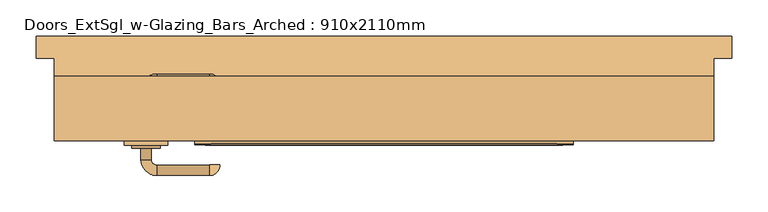
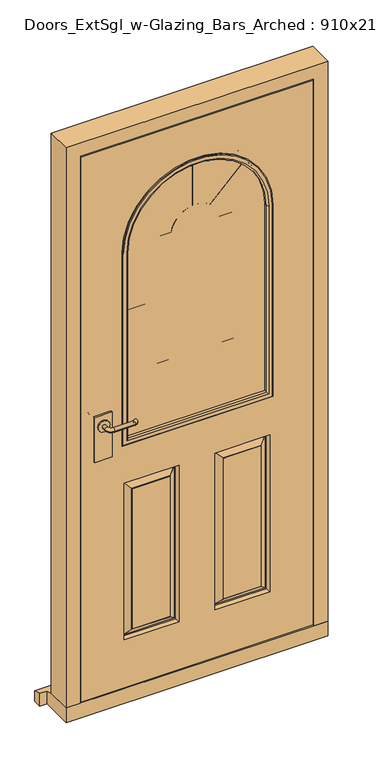
"""IFC4 building model written with IfcOpenShell, lengths in millimetres: door geometry, Doors_ExtSgl_w-Glazing_Bars_Arched : 910x2110mm."""

from ifc_helpers import new_model, si_unit, point, frame, frame_2d, origin, place, context, project, spatial, polyline, circle_curve, ellipse_curve, trimmed, segment, composite_curve, outline, extrude, faceted_brep, source, transform, mapped, element, save
from ifc_brep_helpers import plane_surface, cylinder_surface, revolved_surface, advanced_brep


def doors_extsgl_w_glazing_bars_arched_910x2110mm_1ab485ba(model_context):
    return source(origin(), model_context, "Body", "SolidModel", [
        extrude(outline(composite_curve([segment(trimmed(circle_curve(frame_2d((1050.0, -328.5)), 20.0), [point((1050.0, -348.5))], [point((1050.0, -308.5))], False, "CARTESIAN"), True, "CONTINUOUS"), segment(trimmed(circle_curve(frame_2d((1050.0, -328.5)), 20.0), [point((1050.0, -308.5))], [point((1050.0, -348.5))], False, "CARTESIAN"), True, "CONTINUOUS")], self_intersect=False)), frame((0.0, -22.9929895, 0.0), z_axis=(0.0, 1.0, 0.0), x_axis=(0.0, 0.0, 1.0)), (0.0, 0.0, 1.0), 4.5929895),
        advanced_brep(
        [(-321.5, -22.9929895, 1050.0), (-335.5, -22.9929895, 1050.0), (-335.5, -38.4, 1050.0), (-321.5, -38.4, 1050.0), (-313.5, -60.4, 1050.0), (-313.5, -46.4, 1050.0), (-241.5, -60.4, 1050.0), (-241.5, -46.4, 1050.0), (-240.5, -45.4, 1050.0), (-226.5, -45.4, 1050.0)],
        [
            (0, 1, circle_curve(frame((-328.5, -22.9929895, 1050.0), z_axis=(0.0, 1.0, 0.0), x_axis=(-1.0, 0.0, 0.0)), 7.0)),
            (1, 0, circle_curve(frame((-328.5, -22.9929895, 1050.0), z_axis=(0.0, 1.0, 0.0), x_axis=(-1.0, 0.0, 0.0)), 7.0)),
            (1, 2),
            (2, 3, circle_curve(frame((-328.5, -38.4, 1050.0), z_axis=(0.0, 1.0, 0.0), x_axis=(-1.0, 0.0, 0.0)), 7.0)),
            (3, 0),
            (3, 2, circle_curve(frame((-328.5, -38.4, 1050.0), z_axis=(0.0, 1.0, 0.0), x_axis=(-1.0, 0.0, 0.0)), 7.0)),
            (4, 5, circle_curve(frame((-313.5, -53.4, 1050.0), z_axis=(-1.0, 0.0, 0.0), x_axis=(0.0, -1.0, 0.0)), 7.0)),
            (5, 3, circle_curve(frame((-313.5, -38.4, 1050.0), z_axis=(0.0, 0.0, -1.0), x_axis=(-1.0, 0.0, 0.0)), 8.0)),
            (2, 4, circle_curve(frame((-313.5, -38.4, 1050.0), z_axis=(0.0, 0.0, 1.0), x_axis=(-1.0, 0.0, 0.0)), 22.0)),
            (5, 4, circle_curve(frame((-313.5, -53.4, 1050.0), z_axis=(-1.0, 0.0, 0.0), x_axis=(0.0, -1.0, 0.0)), 7.0)),
            (4, 6),
            (6, 7, circle_curve(frame((-241.5, -53.4, 1050.0), z_axis=(-1.0, 0.0, 0.0), x_axis=(0.0, -1.0, 0.0)), 7.0)),
            (7, 5),
            (7, 6, circle_curve(frame((-241.5, -53.4, 1050.0), z_axis=(-1.0, 0.0, 0.0), x_axis=(0.0, -1.0, 0.0)), 7.0)),
            (8, 9, circle_curve(frame((-233.5, -45.4, 1050.0), z_axis=(0.0, 1.0, 0.0), x_axis=(1.0, 0.0, 0.0)), 7.0)),
            (9, 8, circle_curve(frame((-233.5, -45.4, 1050.0), z_axis=(0.0, 1.0, 0.0), x_axis=(1.0, 0.0, 0.0)), 7.0)),
            (8, 7, circle_curve(frame((-241.5, -45.4, 1050.0), z_axis=(0.0, 0.0, -1.0), x_axis=(0.0, -1.0, 0.0)), 1.0)),
            (6, 9, circle_curve(frame((-241.5, -45.4, 1050.0), z_axis=(0.0, 0.0, 1.0), x_axis=(0.0, -1.0, 0.0)), 15.0)),
        ],
        [
            plane_surface(frame((-328.5, -22.9929895, 1050.0), z_axis=(0.0, 1.0, 0.0), x_axis=(0.0, 0.0, 1.0))),
            cylinder_surface(frame((-328.5, -22.9929895, 1050.0), z_axis=(0.0, 1.0, 0.0), x_axis=(-1.0, 0.0, 0.0)), 7.0),
            revolved_surface(trimmed(ellipse_curve(frame((-328.5, -38.4, 1050.0), z_axis=(0.0, -1.0, 0.0), x_axis=(-1.0, 0.0, 0.0)), 7.0, 7.0), [point((-321.5, -38.4, 1050.0))], [point((-335.5, -38.4, 1050.0))], True, "CARTESIAN"), (-313.5, -38.4, 1050.0), (0.0, 0.0, -1.0)),
            revolved_surface(trimmed(ellipse_curve(frame((-328.5, -38.4, 1050.0), z_axis=(0.0, -1.0, 0.0), x_axis=(-1.0, 0.0, 0.0)), 7.0, 7.0), [point((-335.5, -38.4, 1050.0))], [point((-321.5, -38.4, 1050.0))], True, "CARTESIAN"), (-313.5, -38.4, 1050.0), (0.0, 0.0, -1.0)),
            cylinder_surface(frame((-313.5, -53.4, 1050.0), z_axis=(-1.0, 0.0, 0.0), x_axis=(0.0, -1.0, 0.0)), 7.0),
            plane_surface(frame((-233.5, -45.4, 1050.0), z_axis=(0.0, 1.0, 0.0), x_axis=(0.0, 0.0, 1.0))),
            revolved_surface(trimmed(ellipse_curve(frame((-241.5, -53.4, 1050.0), z_axis=(1.0, 0.0, 0.0), x_axis=(0.0, -1.0, 0.0)), 7.0, 7.0), [point((-241.5, -46.4, 1050.0))], [point((-241.5, -60.4, 1050.0))], True, "CARTESIAN"), (-241.5, -45.4, 1050.0), (0.0, 0.0, -1.0)),
            revolved_surface(trimmed(ellipse_curve(frame((-241.5, -53.4, 1050.0), z_axis=(1.0, 0.0, 0.0), x_axis=(0.0, -1.0, 0.0)), 7.0, 7.0), [point((-241.5, -60.4, 1050.0))], [point((-241.5, -46.4, 1050.0))], True, "CARTESIAN"), (-241.5, -45.4, 1050.0), (0.0, 0.0, -1.0)),
        ],
        [
            (0, [[1, 2]]),
            (1, [[3, 4, 5, -2]]),
            (1, [[-5, 6, -3, -1]]),
            (2, [[7, 8, -4, 9]]),
            (3, [[10, -9, -6, -8]]),
            (4, [[11, 12, 13, -7]]),
            (4, [[-13, 14, -11, -10]]),
            (5, [[15, 16]]),
            (6, [[-15, 17, -12, 18]]),
            (7, [[-16, -18, -14, -17]]),
        ],
    ),
        extrude(outline(polyline([(-298.5, -12.4), (-298.5, -18.4), (-358.5, -18.4), (-358.5, -12.4), (-298.5, -12.4)])), frame((0.0, 0.0, 925.0), z_axis=(0.0, 0.0, 1.0), x_axis=(1.0, 0.0, 0.0)), (0.0, 0.0, 1.0), 165.0),
        extrude(outline(composite_curve([segment(trimmed(circle_curve(frame_2d((1050.0, -328.5)), 20.0), [point((1050.0, -348.5))], [point((1050.0, -308.5))], False, "CARTESIAN"), True, "CONTINUOUS"), segment(trimmed(circle_curve(frame_2d((1050.0, -328.5)), 20.0), [point((1050.0, -308.5))], [point((1050.0, -348.5))], False, "CARTESIAN"), True, "CONTINUOUS")], self_intersect=False)), frame((0.0, 37.6, 0.0), z_axis=(0.0, 1.0, 0.0), x_axis=(0.0, 0.0, 1.0)), (0.0, 0.0, 1.0), 4.5929895),
        advanced_brep(
        [(-321.5, 42.1929895, 1050.0), (-335.5, 42.1929895, 1050.0), (-321.5, 57.6, 1050.0), (-335.5, 57.6, 1050.0), (-313.5, 79.6, 1050.0), (-313.5, 65.6, 1050.0), (-241.5, 65.6, 1050.0), (-241.5, 79.6, 1050.0), (-240.5, 64.6, 1050.0), (-226.5, 64.6, 1050.0)],
        [
            (0, 1, circle_curve(frame((-328.5, 42.1929895, 1050.0), z_axis=(0.0, -1.0, 0.0), x_axis=(-1.0, 0.0, 0.0)), 7.0)),
            (1, 0, circle_curve(frame((-328.5, 42.1929895, 1050.0), z_axis=(0.0, -1.0, 0.0), x_axis=(-1.0, 0.0, 0.0)), 7.0)),
            (0, 2),
            (2, 3, circle_curve(frame((-328.5, 57.6, 1050.0), z_axis=(0.0, -1.0, 0.0), x_axis=(-1.0, 0.0, 0.0)), 7.0)),
            (3, 1),
            (3, 2, circle_curve(frame((-328.5, 57.6, 1050.0), z_axis=(0.0, -1.0, 0.0), x_axis=(-1.0, 0.0, 0.0)), 7.0)),
            (4, 3, circle_curve(frame((-313.5, 57.6, 1050.0), z_axis=(0.0, 0.0, 1.0), x_axis=(-1.0, 0.0, 0.0)), 22.0)),
            (2, 5, circle_curve(frame((-313.5, 57.6, 1050.0), z_axis=(0.0, 0.0, -1.0), x_axis=(-1.0, 0.0, 0.0)), 8.0)),
            (5, 4, circle_curve(frame((-313.5, 72.6, 1050.0), z_axis=(-1.0, 0.0, 0.0), x_axis=(0.0, 1.0, 0.0)), 7.0)),
            (4, 5, circle_curve(frame((-313.5, 72.6, 1050.0), z_axis=(-1.0, 0.0, 0.0), x_axis=(0.0, 1.0, 0.0)), 7.0)),
            (5, 6),
            (6, 7, circle_curve(frame((-241.5, 72.6, 1050.0), z_axis=(-1.0, 0.0, 0.0), x_axis=(0.0, 1.0, 0.0)), 7.0)),
            (7, 4),
            (7, 6, circle_curve(frame((-241.5, 72.6, 1050.0), z_axis=(-1.0, 0.0, 0.0), x_axis=(0.0, 1.0, 0.0)), 7.0)),
            (8, 9, circle_curve(frame((-233.5, 64.6, 1050.0), z_axis=(0.0, -1.0, 0.0), x_axis=(1.0, 0.0, 0.0)), 7.0)),
            (9, 8, circle_curve(frame((-233.5, 64.6, 1050.0), z_axis=(0.0, -1.0, 0.0), x_axis=(1.0, 0.0, 0.0)), 7.0)),
            (9, 7, circle_curve(frame((-241.5, 64.6, 1050.0), z_axis=(0.0, 0.0, 1.0), x_axis=(0.0, 1.0, 0.0)), 15.0)),
            (6, 8, circle_curve(frame((-241.5, 64.6, 1050.0), z_axis=(0.0, 0.0, -1.0), x_axis=(0.0, 1.0, 0.0)), 1.0)),
        ],
        [
            plane_surface(frame((-328.5, 42.1929895, 1050.0), z_axis=(0.0, -1.0, 0.0), x_axis=(0.0, 0.0, 1.0))),
            cylinder_surface(frame((-328.5, 42.1929895, 1050.0), z_axis=(0.0, -1.0, 0.0), x_axis=(-1.0, 0.0, 0.0)), 7.0),
            revolved_surface(trimmed(ellipse_curve(frame((-328.5, 57.6, 1050.0), z_axis=(0.0, -1.0, 0.0), x_axis=(-1.0, 0.0, 0.0)), 7.0, 7.0), [point((-321.5, 57.6, 1050.0))], [point((-335.5, 57.6, 1050.0))], True, "CARTESIAN"), (-313.5, 57.6, 1050.0), (0.0, 0.0, -1.0)),
            revolved_surface(trimmed(ellipse_curve(frame((-328.5, 57.6, 1050.0), z_axis=(0.0, -1.0, 0.0), x_axis=(-1.0, 0.0, 0.0)), 7.0, 7.0), [point((-335.5, 57.6, 1050.0))], [point((-321.5, 57.6, 1050.0))], True, "CARTESIAN"), (-313.5, 57.6, 1050.0), (0.0, 0.0, -1.0)),
            cylinder_surface(frame((-313.5, 72.6, 1050.0), z_axis=(-1.0, 0.0, 0.0), x_axis=(0.0, 1.0, 0.0)), 7.0),
            plane_surface(frame((-233.5, 64.6, 1050.0), z_axis=(0.0, -1.0, 0.0), x_axis=(0.0, 0.0, 1.0))),
            revolved_surface(trimmed(ellipse_curve(frame((-241.5, 72.6, 1050.0), z_axis=(-1.0, 0.0, 0.0), x_axis=(0.0, 1.0, 0.0)), 7.0, 7.0), [point((-241.5, 65.6, 1050.0))], [point((-241.5, 79.6, 1050.0))], True, "CARTESIAN"), (-241.5, 64.6, 1050.0), (0.0, 0.0, -1.0)),
            revolved_surface(trimmed(ellipse_curve(frame((-241.5, 72.6, 1050.0), z_axis=(-1.0, 0.0, 0.0), x_axis=(0.0, 1.0, 0.0)), 7.0, 7.0), [point((-241.5, 79.6, 1050.0))], [point((-241.5, 65.6, 1050.0))], True, "CARTESIAN"), (-241.5, 64.6, 1050.0), (0.0, 0.0, -1.0)),
        ],
        [
            (0, [[1, 2]]),
            (1, [[-1, 3, 4, 5]]),
            (1, [[-2, -5, 6, -3]]),
            (2, [[7, -4, 8, 9]]),
            (3, [[-8, -6, -7, 10]]),
            (4, [[-9, 11, 12, 13]]),
            (4, [[-10, -13, 14, -11]]),
            (5, [[15, 16]]),
            (6, [[17, -12, 18, -16]]),
            (7, [[-18, -14, -17, -15]]),
        ],
    ),
        extrude(outline(polyline([(-298.5, 31.6), (-358.5, 31.6), (-358.5, 37.6), (-298.5, 37.6), (-298.5, 31.6)])), frame((0.0, 0.0, 925.0), z_axis=(0.0, 0.0, 1.0), x_axis=(1.0, 0.0, 0.0)), (0.0, 0.0, 1.0), 165.0),
        faceted_brep([(384.5, 76.6, 54.5), (455.0, 76.6, 54.5), (455.0, -12.4, 54.5), (406.5, -12.4, 54.5), (406.5, 34.6, 54.5), (384.5, 34.6, 54.5), (384.5, 76.6, 2039.5), (-384.5, 76.6, 2039.5), (-384.5, 76.6, 54.5), (-455.0, 76.6, 54.5), (-455.0, 76.6, 2110.0), (455.0, 76.6, 2110.0), (455.0, -12.4, 2110.0), (-455.0, -12.4, 2110.0), (-455.0, -12.4, 54.5), (-406.5, -12.4, 54.5), (-406.5, -12.4, 2061.5), (406.5, -12.4, 2061.5), (406.5, 34.6, 2061.5), (-406.5, 34.6, 2061.5), (-406.5, 34.6, 54.5), (-384.5, 34.6, 54.5), (-384.5, 34.6, 2039.5), (384.5, 34.6, 2039.5)], [[[0, 1, 2, 3, 4, 5]], [[1, 0, 6, 7, 8, 9, 10, 11]], [[2, 1, 11, 12]], [[3, 2, 12, 13, 14, 15, 16, 17]], [[4, 3, 17, 18]], [[5, 4, 18, 19, 20, 21, 22, 23]], [[0, 5, 23, 6]], [[8, 7, 22, 21]], [[9, 8, 21, 20, 15, 14]], [[10, 9, 14, 13]], [[16, 15, 20, 19]], [[11, 10, 13, 12]], [[17, 16, 19, 18]], [[7, 6, 23, 22]]]),
        advanced_brep(
        [(403.5, -12.4, 58.5), (403.5, -12.4, 2058.5), (-404.4250294, -12.4, 2058.5), (-404.4250294, -12.4, 58.5), (-253.5, -12.4, 958.5), (-253.5, -12.4, 1655.0), (253.5, -12.4, 1655.0), (253.5, -12.4, 958.5), (-62.5, -12.4, 808.5), (-62.5, -12.4, 233.5), (-253.5, -12.4, 233.5), (-253.5, -12.4, 808.5), (253.5, -12.4, 808.5), (253.5, -12.4, 233.5), (62.5, -12.4, 233.5), (62.5, -12.4, 808.5), (-92.5, -12.4, 263.5), (-92.5, -12.4, 778.5), (-223.5, -12.4, 778.5), (-223.5, -12.4, 263.5), (223.5, -12.4, 263.5), (223.5, -12.4, 778.5), (92.5, -12.4, 778.5), (92.5, -12.4, 263.5), (403.5, 31.6, 58.5), (-404.4250294, 31.6, 58.5), (-404.4250294, 31.6, 2058.5), (403.5, 31.6, 2058.5), (-253.5, 31.6, 958.5), (253.5, 31.6, 958.5), (253.5, 31.6, 1655.0), (-253.5, 31.6, 1655.0), (62.5, 31.6, 808.5), (62.5, 31.6, 233.5), (253.5, 31.6, 233.5), (253.5, 31.6, 808.5), (-253.5, 31.6, 808.5), (-253.5, 31.6, 233.5), (-62.5, 31.6, 233.5), (-62.5, 31.6, 808.5), (92.5, 31.6, 263.5), (92.5, 31.6, 778.5), (223.5, 31.6, 778.5), (223.5, 31.6, 263.5), (-223.5, 31.6, 263.5), (-223.5, 31.6, 778.5), (-92.5, 31.6, 778.5), (-92.5, 31.6, 263.5), (65.5, 16.6, 805.5), (65.5, 16.6, 236.5), (90.5, 30.6, 780.5), (90.5, 30.6, 261.5), (70.5, 16.6, 241.5), (70.5, 16.6, 800.5), (92.5, 30.6, 263.5), (92.5, 30.6, 778.5), (250.5, 16.6, 236.5), (225.5, 30.6, 261.5), (245.5, 16.6, 241.5), (223.5, 30.6, 263.5), (250.5, 16.6, 805.5), (225.5, 30.6, 780.5), (245.5, 16.6, 800.5), (223.5, 30.6, 778.5), (-250.5, 16.6, 805.5), (-250.5, 16.6, 236.5), (-225.5, 30.6, 780.5), (-225.5, 30.6, 261.5), (-245.5, 16.6, 241.5), (-245.5, 16.6, 800.5), (-223.5, 30.6, 263.5), (-223.5, 30.6, 778.5), (-65.5, 16.6, 236.5), (-90.5, 30.6, 261.5), (-70.5, 16.6, 241.5), (-92.5, 30.6, 263.5), (-65.5, 16.6, 805.5), (-90.5, 30.6, 780.5), (-70.5, 16.6, 800.5), (-92.5, 30.6, 778.5), (-92.5, -11.4, 263.5), (-92.5, -11.4, 778.5), (-70.5, 2.6, 241.5), (-70.5, 2.6, 800.5), (-90.5, -11.4, 780.5), (-90.5, -11.4, 261.5), (-65.5, 2.6, 805.5), (-65.5, 2.6, 236.5), (-223.5, -11.4, 778.5), (-245.5, 2.6, 800.5), (-225.5, -11.4, 780.5), (-250.5, 2.6, 805.5), (-223.5, -11.4, 263.5), (-245.5, 2.6, 241.5), (-225.5, -11.4, 261.5), (-250.5, 2.6, 236.5), (250.5, 2.6, 805.5), (250.5, 2.6, 236.5), (225.5, -11.4, 780.5), (225.5, -11.4, 261.5), (245.5, 2.6, 241.5), (245.5, 2.6, 800.5), (223.5, -11.4, 263.5), (223.5, -11.4, 778.5), (65.5, 2.6, 236.5), (90.5, -11.4, 261.5), (70.5, 2.6, 241.5), (92.5, -11.4, 263.5), (65.5, 2.6, 805.5), (90.5, -11.4, 780.5), (70.5, 2.6, 800.5), (92.5, -11.4, 778.5)],
        [
            (0, 1),
            (1, 2),
            (2, 3),
            (3, 0),
            (4, 5),
            (5, 6, circle_curve(frame((0.0, -12.4, 1655.0), z_axis=(0.0, 1.0, 0.0), x_axis=(1.0, 0.0, 0.0)), 253.5)),
            (6, 7),
            (7, 4),
            (8, 9),
            (9, 10),
            (10, 11),
            (11, 8),
            (12, 13),
            (13, 14),
            (14, 15),
            (15, 12),
            (16, 17),
            (17, 18),
            (18, 19),
            (19, 16),
            (20, 21),
            (21, 22),
            (22, 23),
            (23, 20),
            (24, 25),
            (25, 26),
            (26, 27),
            (27, 24),
            (28, 29),
            (29, 30),
            (30, 31, circle_curve(frame((0.0, 31.6, 1655.0), z_axis=(0.0, -1.0, 0.0), x_axis=(1.0, 0.0, 0.0)), 253.5)),
            (31, 28),
            (32, 33),
            (33, 34),
            (34, 35),
            (35, 32),
            (36, 37),
            (37, 38),
            (38, 39),
            (39, 36),
            (40, 41),
            (41, 42),
            (42, 43),
            (43, 40),
            (44, 45),
            (45, 46),
            (46, 47),
            (47, 44),
            (0, 24),
            (27, 1),
            (26, 2),
            (25, 3),
            (4, 28),
            (31, 5),
            (30, 6),
            (29, 7),
            (48, 49),
            (49, 33),
            (32, 48),
            (50, 51),
            (51, 52),
            (52, 53),
            (53, 50),
            (40, 54),
            (54, 55),
            (55, 41),
            (49, 56),
            (56, 34),
            (51, 57),
            (57, 58),
            (58, 52),
            (43, 59),
            (59, 54),
            (56, 60),
            (60, 35),
            (57, 61),
            (61, 62),
            (62, 58),
            (42, 63),
            (63, 59),
            (60, 48),
            (62, 53),
            (61, 50),
            (63, 55),
            (64, 65),
            (65, 37),
            (36, 64),
            (66, 67),
            (67, 68),
            (68, 69),
            (69, 66),
            (44, 70),
            (70, 71),
            (71, 45),
            (65, 72),
            (72, 38),
            (67, 73),
            (73, 74),
            (74, 68),
            (47, 75),
            (75, 70),
            (72, 76),
            (76, 39),
            (73, 77),
            (77, 78),
            (78, 74),
            (46, 79),
            (79, 75),
            (76, 64),
            (78, 69),
            (77, 66),
            (79, 71),
            (80, 81),
            (81, 17),
            (16, 80),
            (82, 83),
            (83, 84),
            (84, 85),
            (85, 82),
            (8, 86),
            (86, 87),
            (87, 9),
            (81, 88),
            (88, 18),
            (83, 89),
            (89, 90),
            (90, 84),
            (11, 91),
            (91, 86),
            (88, 92),
            (92, 19),
            (89, 93),
            (93, 94),
            (94, 90),
            (10, 95),
            (95, 91),
            (92, 80),
            (94, 85),
            (93, 82),
            (95, 87),
            (96, 97),
            (97, 13),
            (12, 96),
            (98, 99),
            (99, 100),
            (100, 101),
            (101, 98),
            (20, 102),
            (102, 103),
            (103, 21),
            (97, 104),
            (104, 14),
            (99, 105),
            (105, 106),
            (106, 100),
            (23, 107),
            (107, 102),
            (104, 108),
            (108, 15),
            (105, 109),
            (109, 110),
            (110, 106),
            (22, 111),
            (111, 107),
            (108, 96),
            (110, 101),
            (109, 98),
            (111, 103),
        ],
        [
            plane_surface(frame((403.5, -12.4, 58.5), z_axis=(0.0, -1.0, 0.0), x_axis=(0.0, 0.0, 1.0))),
            plane_surface(frame((403.5, 31.6, 58.5), z_axis=(0.0, 1.0, 0.0), x_axis=(0.0, 0.0, -1.0))),
            plane_surface(frame((403.5, -12.4, 58.5), z_axis=(1.0, 0.0, 0.0), x_axis=(0.0, 1.0, 0.0))),
            plane_surface(frame((403.5, -12.4, 2058.5), z_axis=(0.0, 0.0, 1.0), x_axis=(0.0, 1.0, 0.0))),
            plane_surface(frame((-404.4250294, -12.4, 2058.5), z_axis=(-1.0, 0.0, 0.0), x_axis=(0.0, 1.0, 0.0))),
            plane_surface(frame((-404.4250294, -12.4, 58.5), z_axis=(0.0, 0.0, -1.0), x_axis=(0.0, 1.0, 0.0))),
            plane_surface(frame((-253.5, -12.4, 958.5), z_axis=(1.0, 0.0, 0.0), x_axis=(0.0, 1.0, 0.0))),
            revolved_surface(polyline([(253.5, 31.6, 1655.0), (253.5, -12.4, 1655.0)]), (0.0, -12.4, 1655.0), (0.0, 1.0, 0.0)),
            plane_surface(frame((253.5, -12.4, 1655.0), z_axis=(-1.0, 0.0, 0.0), x_axis=(0.0, 1.0, 0.0))),
            plane_surface(frame((253.5, -12.4, 958.5), z_axis=(0.0, 0.0, 1.0), x_axis=(0.0, 1.0, 0.0))),
            plane_surface(frame((62.5, 31.6, 808.5), z_axis=(0.9805806756909202, 0.19611613513818407, 0.0), x_axis=(0.0, 0.0, -1.0))),
            plane_surface(frame((70.5, 16.6, 800.5), z_axis=(-0.5734623443633278, 0.8192319205190408, 0.0), x_axis=(0.0, 0.0, -1.0))),
            plane_surface(frame((92.5, 30.6, 778.5), z_axis=(-1.0, 0.0, 0.0), x_axis=(0.0, 0.0, -1.0))),
            plane_surface(frame((62.5, 31.6, 233.5), z_axis=(0.0, 0.19611613513818724, 0.9805806756909196), x_axis=(1.0, 0.0, 0.0))),
            plane_surface(frame((70.5, 16.6, 241.5), z_axis=(0.0, 0.819231920519039, -0.5734623443633305), x_axis=(1.0, 0.0, 0.0))),
            plane_surface(frame((92.5, 30.6, 263.5), z_axis=(0.0, 0.0, -1.0), x_axis=(1.0, 0.0, 0.0))),
            plane_surface(frame((253.5, 31.6, 233.5), z_axis=(-0.9805806756909189, 0.19611613513819037, 0.0), x_axis=(0.0, 0.0, 1.0))),
            plane_surface(frame((245.5, 16.6, 241.5), z_axis=(0.5734623443633332, 0.819231920519037, 0.0), x_axis=(0.0, 0.0, 1.0))),
            plane_surface(frame((223.5, 30.6, 263.5), z_axis=(1.0, 0.0, 0.0), x_axis=(0.0, 0.0, 1.0))),
            plane_surface(frame((253.5, 31.6, 808.5), z_axis=(0.0, 0.1961161351381872, -0.9805806756909196), x_axis=(-1.0, 0.0, 0.0))),
            plane_surface(frame((250.5, 16.6, 805.5), z_axis=(0.0, 1.0, 0.0), x_axis=(-1.0, 0.0, 0.0))),
            plane_surface(frame((245.5, 16.6, 800.5), z_axis=(0.0, 0.8192319205190389, 0.5734623443633305), x_axis=(-1.0, 0.0, 0.0))),
            plane_surface(frame((225.5, 30.6, 780.5), z_axis=(0.0, 1.0, 0.0), x_axis=(-1.0, 0.0, 0.0))),
            plane_surface(frame((223.5, 30.6, 778.5), z_axis=(0.0, 0.0, 1.0), x_axis=(-1.0, 0.0, 0.0))),
            plane_surface(frame((-253.5, 31.6, 808.5), z_axis=(0.9805806756909202, 0.19611613513818407, 0.0), x_axis=(0.0, 0.0, -1.0))),
            plane_surface(frame((-245.5, 16.6, 800.5), z_axis=(-0.5734623443633278, 0.8192319205190408, 0.0), x_axis=(0.0, 0.0, -1.0))),
            plane_surface(frame((-223.5, 30.6, 778.5), z_axis=(-1.0, 0.0, 0.0), x_axis=(0.0, 0.0, -1.0))),
            plane_surface(frame((-253.5, 31.6, 233.5), z_axis=(0.0, 0.19611613513818724, 0.9805806756909196), x_axis=(1.0, 0.0, 0.0))),
            plane_surface(frame((-245.5, 16.6, 241.5), z_axis=(0.0, 0.819231920519039, -0.5734623443633305), x_axis=(1.0, 0.0, 0.0))),
            plane_surface(frame((-223.5, 30.6, 263.5), z_axis=(0.0, 0.0, -1.0), x_axis=(1.0, 0.0, 0.0))),
            plane_surface(frame((-62.5, 31.6, 233.5), z_axis=(-0.9805806756909189, 0.1961161351381904, 0.0), x_axis=(0.0, 0.0, 1.0))),
            plane_surface(frame((-70.5, 16.6, 241.5), z_axis=(0.5734623443633332, 0.8192319205190371, 0.0), x_axis=(0.0, 0.0, 1.0))),
            plane_surface(frame((-92.5, 30.6, 263.5), z_axis=(1.0, 0.0, 0.0), x_axis=(0.0, 0.0, 1.0))),
            plane_surface(frame((-62.5, 31.6, 808.5), z_axis=(0.0, 0.19611613513818724, -0.9805806756909196), x_axis=(-1.0, 0.0, 0.0))),
            plane_surface(frame((-65.5, 16.6, 805.5), z_axis=(0.0, 1.0, 0.0), x_axis=(-1.0, 0.0, 0.0))),
            plane_surface(frame((-70.5, 16.6, 800.5), z_axis=(0.0, 0.819231920519039, 0.5734623443633305), x_axis=(-1.0, 0.0, 0.0))),
            plane_surface(frame((-90.5, 30.6, 780.5), z_axis=(0.0, 1.0, 0.0), x_axis=(-1.0, 0.0, 0.0))),
            plane_surface(frame((-92.5, 30.6, 778.5), z_axis=(0.0, 0.0, 1.0), x_axis=(-1.0, 0.0, 0.0))),
            plane_surface(frame((-92.5, -12.4, 263.5), z_axis=(1.0, 0.0, 0.0), x_axis=(0.0, 0.0, 1.0))),
            plane_surface(frame((-90.5, -11.4, 261.5), z_axis=(0.5734623443633226, -0.8192319205190446, 0.0), x_axis=(0.0, 0.0, 1.0))),
            plane_surface(frame((-65.5, 2.6, 236.5), z_axis=(-0.9805806756909214, -0.19611613513817774, 0.0), x_axis=(0.0, 0.0, 1.0))),
            plane_surface(frame((-92.5, -12.4, 778.5), z_axis=(0.0, 0.0, 1.0), x_axis=(-1.0, 0.0, 0.0))),
            plane_surface(frame((-90.5, -11.4, 780.5), z_axis=(0.0, -0.8192319205190427, 0.5734623443633252), x_axis=(-1.0, 0.0, 0.0))),
            plane_surface(frame((-65.5, 2.6, 805.5), z_axis=(0.0, -0.1961161351381809, -0.9805806756909208), x_axis=(-1.0, 0.0, 0.0))),
            plane_surface(frame((-223.5, -12.4, 778.5), z_axis=(-1.0, 0.0, 0.0), x_axis=(0.0, 0.0, -1.0))),
            plane_surface(frame((-225.5, -11.4, 780.5), z_axis=(-0.5734623443633279, -0.8192319205190408, 0.0), x_axis=(0.0, 0.0, -1.0))),
            plane_surface(frame((-250.5, 2.6, 805.5), z_axis=(0.9805806756909202, -0.1961161351381841, 0.0), x_axis=(0.0, 0.0, -1.0))),
            plane_surface(frame((-223.5, -12.4, 263.5), z_axis=(0.0, 0.0, -1.0), x_axis=(1.0, 0.0, 0.0))),
            plane_surface(frame((-223.5, -11.4, 263.5), z_axis=(0.0, -1.0, 0.0), x_axis=(1.0, 0.0, 0.0))),
            plane_surface(frame((-225.5, -11.4, 261.5), z_axis=(0.0, -0.8192319205190427, -0.5734623443633252), x_axis=(1.0, 0.0, 0.0))),
            plane_surface(frame((-245.5, 2.6, 241.5), z_axis=(0.0, -1.0, 0.0), x_axis=(1.0, 0.0, 0.0))),
            plane_surface(frame((-250.5, 2.6, 236.5), z_axis=(0.0, -0.19611613513818094, 0.9805806756909209), x_axis=(1.0, 0.0, 0.0))),
            plane_surface(frame((253.5, -12.4, 808.5), z_axis=(-0.9805806756909202, -0.19611613513818407, 0.0), x_axis=(0.0, 0.0, -1.0))),
            plane_surface(frame((245.5, 2.6, 800.5), z_axis=(0.5734623443633278, -0.8192319205190408, 0.0), x_axis=(0.0, 0.0, -1.0))),
            plane_surface(frame((223.5, -11.4, 778.5), z_axis=(1.0, 0.0, 0.0), x_axis=(0.0, 0.0, -1.0))),
            plane_surface(frame((253.5, -12.4, 233.5), z_axis=(0.0, -0.19611613513818724, 0.9805806756909196), x_axis=(-1.0, 0.0, 0.0))),
            plane_surface(frame((245.5, 2.6, 241.5), z_axis=(0.0, -0.819231920519039, -0.5734623443633305), x_axis=(-1.0, 0.0, 0.0))),
            plane_surface(frame((223.5, -11.4, 263.5), z_axis=(0.0, 0.0, -1.0), x_axis=(-1.0, 0.0, 0.0))),
            plane_surface(frame((62.5, -12.4, 233.5), z_axis=(0.9805806756909189, -0.19611613513819046, 0.0), x_axis=(0.0, 0.0, 1.0))),
            plane_surface(frame((70.5, 2.6, 241.5), z_axis=(-0.5734623443633331, -0.8192319205190371, 0.0), x_axis=(0.0, 0.0, 1.0))),
            plane_surface(frame((92.5, -11.4, 263.5), z_axis=(-1.0, 0.0, 0.0), x_axis=(0.0, 0.0, 1.0))),
            plane_surface(frame((62.5, -12.4, 808.5), z_axis=(0.0, -0.1961161351381873, -0.9805806756909196), x_axis=(1.0, 0.0, 0.0))),
            plane_surface(frame((65.5, 2.6, 805.5), z_axis=(0.0, -1.0, 0.0), x_axis=(1.0, 0.0, 0.0))),
            plane_surface(frame((70.5, 2.6, 800.5), z_axis=(0.0, -0.819231920519039, 0.5734623443633304), x_axis=(1.0, 0.0, 0.0))),
            plane_surface(frame((90.5, -11.4, 780.5), z_axis=(0.0, -1.0, 0.0), x_axis=(1.0, 0.0, 0.0))),
            plane_surface(frame((92.5, -11.4, 778.5), z_axis=(0.0, 0.0, 1.0), x_axis=(1.0, 0.0, 0.0))),
        ],
        [
            (0, [[1, 2, 3, 4], [5, 6, 7, 8], [9, 10, 11, 12], [13, 14, 15, 16]]),
            (0, [[17, 18, 19, 20]]),
            (0, [[21, 22, 23, 24]]),
            (1, [[25, 26, 27, 28], [29, 30, 31, 32], [33, 34, 35, 36], [37, 38, 39, 40]]),
            (1, [[41, 42, 43, 44]]),
            (1, [[45, 46, 47, 48]]),
            (2, [[-1, 49, -28, 50]]),
            (3, [[-2, -50, -27, 51]]),
            (4, [[-3, -51, -26, 52]]),
            (5, [[-4, -52, -25, -49]]),
            (6, [[-5, 53, -32, 54]]),
            (7, [[-6, -54, -31, 55]]),
            (8, [[-7, -55, -30, 56]]),
            (9, [[-8, -56, -29, -53]]),
            (10, [[57, 58, -33, 59]]),
            (11, [[60, 61, 62, 63]]),
            (12, [[64, 65, 66, -41]]),
            (13, [[-58, 67, 68, -34]]),
            (14, [[-61, 69, 70, 71]]),
            (15, [[-64, -44, 72, 73]]),
            (16, [[-68, 74, 75, -35]]),
            (17, [[-70, 76, 77, 78]]),
            (18, [[-72, -43, 79, 80]]),
            (19, [[-59, -36, -75, 81]]),
            (20, [[-57, -81, -74, -67], [-62, -71, -78, 82]]),
            (21, [[-63, -82, -77, 83]]),
            (22, [[-60, -83, -76, -69], [-65, -73, -80, 84]]),
            (23, [[-66, -84, -79, -42]]),
            (24, [[85, 86, -37, 87]]),
            (25, [[88, 89, 90, 91]]),
            (26, [[92, 93, 94, -45]]),
            (27, [[-86, 95, 96, -38]]),
            (28, [[-89, 97, 98, 99]]),
            (29, [[-92, -48, 100, 101]]),
            (30, [[-96, 102, 103, -39]]),
            (31, [[-98, 104, 105, 106]]),
            (32, [[-100, -47, 107, 108]]),
            (33, [[-87, -40, -103, 109]]),
            (34, [[-85, -109, -102, -95], [-90, -99, -106, 110]]),
            (35, [[-91, -110, -105, 111]]),
            (36, [[-88, -111, -104, -97], [-93, -101, -108, 112]]),
            (37, [[-94, -112, -107, -46]]),
            (38, [[113, 114, -17, 115]]),
            (39, [[116, 117, 118, 119]]),
            (40, [[120, 121, 122, -9]]),
            (41, [[-114, 123, 124, -18]]),
            (42, [[-117, 125, 126, 127]]),
            (43, [[-120, -12, 128, 129]]),
            (44, [[-124, 130, 131, -19]]),
            (45, [[-126, 132, 133, 134]]),
            (46, [[-128, -11, 135, 136]]),
            (47, [[-115, -20, -131, 137]]),
            (48, [[-118, -127, -134, 138], [-113, -137, -130, -123]]),
            (49, [[-119, -138, -133, 139]]),
            (50, [[-121, -129, -136, 140], [-116, -139, -132, -125]]),
            (51, [[-122, -140, -135, -10]]),
            (52, [[141, 142, -13, 143]]),
            (53, [[144, 145, 146, 147]]),
            (54, [[148, 149, 150, -21]]),
            (55, [[-142, 151, 152, -14]]),
            (56, [[-145, 153, 154, 155]]),
            (57, [[-148, -24, 156, 157]]),
            (58, [[-152, 158, 159, -15]]),
            (59, [[-154, 160, 161, 162]]),
            (60, [[-156, -23, 163, 164]]),
            (61, [[-143, -16, -159, 165]]),
            (62, [[-141, -165, -158, -151], [-146, -155, -162, 166]]),
            (63, [[-147, -166, -161, 167]]),
            (64, [[-144, -167, -160, -153], [-149, -157, -164, 168]]),
            (65, [[-150, -168, -163, -22]]),
        ],
    ),
        faceted_brep([(480.0, 131.6, 0.0), (480.0, 131.6, 38.5947221), (480.0, 101.6, 47.2703282), (480.0, 101.6, 0.0), (-480.0, 131.6, 38.5947221), (-480.0, 131.6, 0.0), (-480.0, 101.6, 0.0), (-480.0, 101.6, 47.2703282), (455.0, 101.6, 0.0), (455.0, -12.4, 0.0), (-455.0, -12.4, 0.0), (-455.0, 101.6, 0.0), (-455.0, 101.6, 47.2703282), (-455.0, 76.6, 54.5), (455.0, 76.6, 54.5), (455.0, 101.6, 47.2703282), (-455.0, -12.4, 54.5), (455.0, -12.4, 54.5)], [[[0, 1, 2, 3]], [[4, 5, 6, 7]], [[5, 0, 3, 8, 9, 10, 11, 6]], [[1, 0, 5, 4]], [[1, 4, 7, 12, 13, 14, 15, 2]], [[13, 16, 17, 14]], [[16, 10, 9, 17]], [[12, 11, 10, 16, 13]], [[11, 12, 7, 6]], [[8, 15, 14, 17, 9]], [[15, 8, 3, 2]]]),
        extrude(outline(composite_curve([segment(polyline([(958.5, -253.5), (958.5, 253.5), (1655.0, 253.5)]), True, "CONTINUOUS"), segment(trimmed(circle_curve(frame_2d((1655.0, 0.0)), 253.5), [point((1655.0, 253.5))], [point((1655.0, -253.5))], False, "CARTESIAN"), True, "CONTINUOUS"), segment(polyline([(1655.0, -253.5), (958.5, -253.5)]), True, "CONTINUOUS")], self_intersect=False)), frame((0.0, -2.4, 0.0), z_axis=(0.0, 1.0, 0.0), x_axis=(0.0, 0.0, 1.0)), (0.0, 0.0, 1.0), 24.0),
        advanced_brep(
        [(-261.5, 35.6, 950.5), (-261.5, 31.6, 950.5), (-261.5, 31.6, 1655.0), (-261.5, 35.6, 1655.0), (-259.5, 37.6, 952.5), (-259.5, 37.6, 1655.0), (-241.5, 32.6, 970.5), (-246.5, 37.6, 965.5), (-246.5, 37.6, 1655.0), (-241.5, 32.6, 1655.0), (-241.5, 21.6, 970.5), (-241.5, 21.6, 1655.0), (-253.5, 31.6, 958.5), (-253.5, 21.6, 958.5), (-253.5, 21.6, 1655.0), (-253.5, 31.6, 1655.0), (261.5, 35.6, 1655.0), (261.5, 31.6, 1655.0), (259.5, 37.6, 1655.0), (259.5, 37.6, 952.5), (246.5, 37.6, 1655.0), (246.5, 37.6, 965.5), (241.5, 32.6, 1655.0), (241.5, 21.6, 1655.0), (253.5, 21.6, 1655.0), (253.5, 21.6, 958.5), (241.5, 21.6, 970.5), (253.5, 31.6, 1655.0), (261.5, 31.6, 950.5), (253.5, 31.6, 958.5), (261.5, 35.6, 950.5), (241.5, 32.6, 970.5)],
        [
            (0, 1),
            (1, 2),
            (2, 3),
            (3, 0),
            (4, 0, ellipse_curve(frame((-259.5, 35.6, 952.5), z_axis=(-0.7071067811865475, 0.0, 0.7071067811865475), x_axis=(-0.7071067811865472, 0.0, -0.7071067811865477)), 2.8284271, 2.0)),
            (3, 5, circle_curve(frame((-259.5, 35.6, 1655.0), z_axis=(0.0, 0.0, -1.0), x_axis=(-1.0, 0.0, 0.0)), 2.0)),
            (5, 4),
            (6, 7, ellipse_curve(frame((-246.5, 32.6, 965.5), z_axis=(-0.7071067811865475, 0.0, 0.7071067811865475), x_axis=(-0.7071067811865472, 0.0, -0.7071067811865477)), 7.0710678, 5.0)),
            (7, 8),
            (8, 9, circle_curve(frame((-246.5, 32.6, 1655.0), z_axis=(0.0, 0.0, -1.0), x_axis=(-1.0, 0.0, 0.0)), 5.0)),
            (9, 6),
            (10, 6),
            (9, 11),
            (11, 10),
            (12, 13),
            (13, 14),
            (14, 15),
            (15, 12),
            (16, 3, circle_curve(frame((0.0, 35.6, 1655.0), z_axis=(0.0, -1.0, 0.0), x_axis=(-1.0, 0.0, 0.0)), 261.5)),
            (2, 17, circle_curve(frame((0.0, 31.6, 1655.0), z_axis=(0.0, 1.0, 0.0), x_axis=(-1.0, 0.0, 0.0)), 261.5)),
            (17, 16),
            (18, 5, circle_curve(frame((0.0, 37.6, 1655.0), z_axis=(0.0, -1.0, 0.0), x_axis=(-1.0, 0.0, 0.0)), 259.5)),
            (16, 18, circle_curve(frame((259.5, 35.6, 1655.0), z_axis=(0.0, 0.0, 1.0), x_axis=(1.0, 0.0, 0.0)), 2.0)),
            (18, 19),
            (19, 4),
            (20, 8, circle_curve(frame((0.0, 37.6, 1655.0), z_axis=(0.0, -1.0, 0.0), x_axis=(-1.0, 0.0, 0.0)), 246.5)),
            (7, 21),
            (21, 20),
            (22, 9, circle_curve(frame((0.0, 32.6, 1655.0), z_axis=(0.0, -1.0, 0.0), x_axis=(-1.0, 0.0, 0.0)), 241.5)),
            (20, 22, circle_curve(frame((246.5, 32.6, 1655.0), z_axis=(0.0, 0.0, 1.0), x_axis=(1.0, 0.0, 0.0)), 5.0)),
            (23, 11, circle_curve(frame((0.0, 21.6, 1655.0), z_axis=(0.0, -1.0, 0.0), x_axis=(-1.0, 0.0, 0.0)), 241.5)),
            (22, 23),
            (24, 14, circle_curve(frame((0.0, 21.6, 1655.0), z_axis=(0.0, -1.0, 0.0), x_axis=(-1.0, 0.0, 0.0)), 253.5)),
            (13, 25),
            (25, 24),
            (23, 26),
            (26, 10),
            (27, 15, circle_curve(frame((0.0, 31.6, 1655.0), z_axis=(0.0, -1.0, 0.0), x_axis=(-1.0, 0.0, 0.0)), 253.5)),
            (24, 27),
            (1, 28),
            (28, 17),
            (27, 29),
            (29, 12),
            (28, 30),
            (30, 16),
            (30, 19, ellipse_curve(frame((259.5, 35.6, 952.5), z_axis=(0.7071067811865475, 0.0, 0.7071067811865475), x_axis=(-0.7071067811865475, 0.0, 0.7071067811865476)), 2.8284271, 2.0)),
            (21, 31, ellipse_curve(frame((246.5, 32.6, 965.5), z_axis=(0.7071067811865475, 0.0, 0.7071067811865475), x_axis=(-0.7071067811865475, 0.0, 0.7071067811865476)), 7.0710678, 5.0)),
            (31, 22),
            (31, 26),
            (25, 29),
            (0, 30),
            (6, 31),
        ],
        [
            plane_surface(frame((-261.5, 31.6, 950.5), z_axis=(-1.0, 0.0, 0.0), x_axis=(0.0, 0.0, 1.0))),
            cylinder_surface(frame((-259.5, 35.6, 958.5), z_axis=(0.0, 0.0, -1.0), x_axis=(-1.0, 0.0, 0.0)), 2.0),
            cylinder_surface(frame((-246.5, 32.6, 958.5), z_axis=(0.0, 0.0, -1.0), x_axis=(-1.0, 0.0, 0.0)), 5.0),
            plane_surface(frame((-241.5, 32.6, 970.5), z_axis=(1.0, 0.0, 0.0), x_axis=(0.0, 0.0, 1.0))),
            plane_surface(frame((-253.5, 21.6, 958.5), z_axis=(-1.0, 0.0, 0.0), x_axis=(0.0, 0.0, 1.0))),
            cylinder_surface(frame((0.0, 31.6, 1655.0), z_axis=(0.0, 1.0, 0.0), x_axis=(-1.0, 0.0, 0.0)), 261.5),
            revolved_surface(trimmed(ellipse_curve(frame((-259.5, 35.6, 1655.0), z_axis=(0.0, 0.0, -1.0), x_axis=(-1.0, 0.0, 0.0)), 2.0, 2.0), [point((-261.5, 35.6, 1655.0))], [point((-259.5, 37.6, 1655.0))], True, "CARTESIAN"), (0.0, 31.6, 1655.0), (0.0, 1.0, 0.0)),
            plane_surface(frame((0.0, 37.6, 1655.0), z_axis=(0.0, 1.0, 0.0), x_axis=(-1.0, 0.0, 0.0))),
            revolved_surface(trimmed(ellipse_curve(frame((-246.5, 32.6, 1655.0), z_axis=(0.0, 0.0, -1.0), x_axis=(-1.0, 0.0, 0.0)), 5.0, 5.0), [point((-246.5, 37.6, 1655.0))], [point((-241.5, 32.6, 1655.0))], True, "CARTESIAN"), (0.0, 31.6, 1655.0), (0.0, 1.0, 0.0)),
            revolved_surface(polyline([(-241.5, 32.6, 1655.0), (-241.5, 21.6, 1655.0)]), (0.0, 31.6, 1655.0), (0.0, 1.0, 0.0)),
            plane_surface(frame((0.0, 21.6, 1655.0), z_axis=(0.0, -1.0, 0.0), x_axis=(-1.0, 0.0, 0.0))),
            cylinder_surface(frame((0.0, 31.6, 1655.0), z_axis=(0.0, 1.0, 0.0), x_axis=(-1.0, 0.0, 0.0)), 253.5),
            plane_surface(frame((0.0, 31.6, 1655.0), z_axis=(0.0, -1.0, 0.0), x_axis=(-1.0, 0.0, 0.0))),
            plane_surface(frame((261.5, 31.6, 1655.0), z_axis=(1.0, 0.0, 0.0), x_axis=(0.0, 0.0, -1.0))),
            cylinder_surface(frame((259.5, 35.6, 1655.0), z_axis=(0.0, 0.0, 1.0), x_axis=(1.0, 0.0, 0.0)), 2.0),
            cylinder_surface(frame((246.5, 32.6, 1655.0), z_axis=(0.0, 0.0, 1.0), x_axis=(1.0, 0.0, 0.0)), 5.0),
            plane_surface(frame((241.5, 32.6, 1655.0), z_axis=(-1.0, 0.0, 0.0), x_axis=(0.0, 0.0, -1.0))),
            plane_surface(frame((253.5, 21.6, 1655.0), z_axis=(1.0, 0.0, 0.0), x_axis=(0.0, 0.0, -1.0))),
            plane_surface(frame((261.5, 31.6, 950.5), z_axis=(0.0, 0.0, -1.0), x_axis=(-1.0, 0.0, 0.0))),
            cylinder_surface(frame((253.5, 35.6, 952.5), z_axis=(1.0, 0.0, 0.0), x_axis=(0.0, 0.0, -1.0)), 2.0),
            cylinder_surface(frame((253.5, 32.6, 965.5), z_axis=(1.0, 0.0, 0.0), x_axis=(0.0, 0.0, -1.0)), 5.0),
            plane_surface(frame((241.5, 32.6, 970.5), z_axis=(0.0, 0.0, 1.0), x_axis=(-1.0, 0.0, 0.0))),
            plane_surface(frame((253.5, 21.6, 958.5), z_axis=(0.0, 0.0, -1.0), x_axis=(-1.0, 0.0, 0.0))),
        ],
        [
            (0, [[1, 2, 3, 4]]),
            (1, [[5, -4, 6, 7]]),
            (2, [[8, 9, 10, 11]]),
            (3, [[12, -11, 13, 14]]),
            (4, [[15, 16, 17, 18]]),
            (5, [[19, -3, 20, 21]]),
            (6, [[22, -6, -19, 23]]),
            (7, [[24, 25, -7, -22], [26, -9, 27, 28]]),
            (8, [[29, -10, -26, 30]]),
            (9, [[31, -13, -29, 32]]),
            (10, [[33, -16, 34, 35], [36, 37, -14, -31]]),
            (11, [[38, -17, -33, 39]]),
            (12, [[-20, -2, 40, 41], [42, 43, -18, -38]]),
            (13, [[-21, -41, 44, 45]]),
            (14, [[-23, -45, 46, -24]]),
            (15, [[-30, -28, 47, 48]]),
            (16, [[-32, -48, 49, -36]]),
            (17, [[-39, -35, 50, -42]]),
            (18, [[-44, -40, -1, 51]]),
            (19, [[-46, -51, -5, -25]]),
            (20, [[-47, -27, -8, 52]]),
            (21, [[-49, -52, -12, -37]]),
            (22, [[-50, -34, -15, -43]]),
        ],
    ),
        advanced_brep(
        [(261.5, -16.4, 950.5), (261.5, -12.4, 950.5), (261.5, -12.4, 1655.0), (261.5, -16.4, 1655.0), (259.5, -18.4, 952.5), (259.5, -18.4, 1655.0), (241.5, -13.4, 970.5), (246.5, -18.4, 965.5), (246.5, -18.4, 1655.0), (241.5, -13.4, 1655.0), (241.5, -2.4, 970.5), (241.5, -2.4, 1655.0), (253.5, -12.4, 958.5), (253.5, -2.4, 958.5), (253.5, -2.4, 1655.0), (253.5, -12.4, 1655.0), (-261.5, -16.4, 1655.0), (-261.5, -12.4, 1655.0), (-259.5, -18.4, 1655.0), (-259.5, -18.4, 952.5), (-246.5, -18.4, 1655.0), (-246.5, -18.4, 965.5), (-241.5, -13.4, 1655.0), (-241.5, -2.4, 1655.0), (-253.5, -2.4, 1655.0), (-253.5, -2.4, 958.5), (-241.5, -2.4, 970.5), (-253.5, -12.4, 1655.0), (-261.5, -12.4, 950.5), (-253.5, -12.4, 958.5), (-261.5, -16.4, 950.5), (-241.5, -13.4, 970.5)],
        [
            (0, 1),
            (1, 2),
            (2, 3),
            (3, 0),
            (4, 0, ellipse_curve(frame((259.5, -16.4, 952.5), z_axis=(0.7071067811865429, 0.0, 0.707106781186552), x_axis=(0.7071067811865519, 0.0, -0.707106781186543)), 2.8284271, 2.0)),
            (3, 5, circle_curve(frame((259.5, -16.4, 1655.0), z_axis=(0.0, 0.0, -1.0), x_axis=(1.0, 0.0, 0.0)), 2.0)),
            (5, 4),
            (6, 7, ellipse_curve(frame((246.5, -13.4, 965.5), z_axis=(0.7071067811865429, 0.0, 0.707106781186552), x_axis=(0.7071067811865519, 0.0, -0.707106781186543)), 7.0710678, 5.0)),
            (7, 8),
            (8, 9, circle_curve(frame((246.5, -13.4, 1655.0), z_axis=(0.0, 0.0, -1.0), x_axis=(1.0, 0.0, 0.0)), 5.0)),
            (9, 6),
            (10, 6),
            (9, 11),
            (11, 10),
            (12, 13),
            (13, 14),
            (14, 15),
            (15, 12),
            (16, 3, circle_curve(frame((0.0, -16.4, 1655.0), z_axis=(0.0, 1.0, 0.0), x_axis=(1.0, 0.0, 0.0)), 261.5)),
            (2, 17, circle_curve(frame((0.0, -12.4, 1655.0), z_axis=(0.0, -1.0, 0.0), x_axis=(1.0, 0.0, 0.0)), 261.5)),
            (17, 16),
            (18, 5, circle_curve(frame((0.0, -18.4, 1655.0), z_axis=(0.0, 1.0, 0.0), x_axis=(1.0, 0.0, 0.0)), 259.5)),
            (16, 18, circle_curve(frame((-259.5, -16.4, 1655.0), z_axis=(0.0, 0.0, 1.0), x_axis=(-1.0, 0.0, 0.0)), 2.0)),
            (18, 19),
            (19, 4),
            (20, 8, circle_curve(frame((0.0, -18.4, 1655.0), z_axis=(0.0, 1.0, 0.0), x_axis=(1.0, 0.0, 0.0)), 246.5)),
            (7, 21),
            (21, 20),
            (22, 9, circle_curve(frame((0.0, -13.4, 1655.0), z_axis=(0.0, 1.0, 0.0), x_axis=(1.0, 0.0, 0.0)), 241.5)),
            (20, 22, circle_curve(frame((-246.5, -13.4, 1655.0), z_axis=(0.0, 0.0, 1.0), x_axis=(-1.0, 0.0, 0.0)), 5.0)),
            (23, 11, circle_curve(frame((0.0, -2.4, 1655.0), z_axis=(0.0, 1.0, 0.0), x_axis=(1.0, 0.0, 0.0)), 241.5)),
            (22, 23),
            (24, 14, circle_curve(frame((0.0, -2.4, 1655.0), z_axis=(0.0, 1.0, 0.0), x_axis=(1.0, 0.0, 0.0)), 253.5)),
            (13, 25),
            (25, 24),
            (23, 26),
            (26, 10),
            (27, 15, circle_curve(frame((0.0, -12.4, 1655.0), z_axis=(0.0, 1.0, 0.0), x_axis=(1.0, 0.0, 0.0)), 253.5)),
            (24, 27),
            (1, 28),
            (28, 17),
            (27, 29),
            (29, 12),
            (28, 30),
            (30, 16),
            (30, 19, ellipse_curve(frame((-259.5, -16.4, 952.5), z_axis=(-0.707106781186552, 0.0, 0.7071067811865429), x_axis=(0.7071067811865428, 0.0, 0.7071067811865521)), 2.8284271, 2.0)),
            (21, 31, ellipse_curve(frame((-246.5, -13.4, 965.5), z_axis=(-0.707106781186552, 0.0, 0.7071067811865429), x_axis=(0.7071067811865428, 0.0, 0.7071067811865521)), 7.0710678, 5.0)),
            (31, 22),
            (31, 26),
            (25, 29),
            (0, 30),
            (6, 31),
        ],
        [
            plane_surface(frame((261.5, -12.4, 950.5), z_axis=(1.0, 0.0, 0.0), x_axis=(0.0, 0.0, 1.0))),
            cylinder_surface(frame((259.5, -16.4, 958.5), z_axis=(0.0, 0.0, -1.0), x_axis=(1.0, 0.0, 0.0)), 2.0),
            cylinder_surface(frame((246.5, -13.4, 958.5), z_axis=(0.0, 0.0, -1.0), x_axis=(1.0, 0.0, 0.0)), 5.0),
            plane_surface(frame((241.5, -13.4, 970.5), z_axis=(-1.0, 0.0, 0.0), x_axis=(0.0, 0.0, 1.0))),
            plane_surface(frame((253.5, -2.4, 958.5), z_axis=(1.0, 0.0, 0.0), x_axis=(0.0, 0.0, 1.0))),
            cylinder_surface(frame((0.0, -12.4, 1655.0), z_axis=(0.0, -1.0, 0.0), x_axis=(1.0, 0.0, 0.0)), 261.5),
            revolved_surface(trimmed(ellipse_curve(frame((259.5, -16.4, 1655.0), z_axis=(0.0, 0.0, -1.0), x_axis=(1.0, 0.0, 0.0)), 2.0, 2.0), [point((261.5, -16.4, 1655.0))], [point((259.5, -18.4, 1655.0))], True, "CARTESIAN"), (0.0, -12.4, 1655.0), (0.0, -1.0, 0.0)),
            plane_surface(frame((0.0, -18.4, 1655.0), z_axis=(0.0, -1.0, 0.0), x_axis=(1.0, 0.0, 0.0))),
            revolved_surface(trimmed(ellipse_curve(frame((246.5, -13.4, 1655.0), z_axis=(0.0, 0.0, -1.0), x_axis=(1.0, 0.0, 0.0)), 5.0, 5.0), [point((246.5, -18.4, 1655.0))], [point((241.5, -13.4, 1655.0))], True, "CARTESIAN"), (0.0, -12.4, 1655.0), (0.0, -1.0, 0.0)),
            revolved_surface(polyline([(241.5, -13.4, 1655.0), (241.5, -2.4000000000000004, 1655.0)]), (0.0, -12.4, 1655.0), (0.0, -1.0, 0.0)),
            plane_surface(frame((0.0, -2.4, 1655.0), z_axis=(0.0, 1.0, 0.0), x_axis=(1.0, 0.0, 0.0))),
            cylinder_surface(frame((0.0, -12.4, 1655.0), z_axis=(0.0, -1.0, 0.0), x_axis=(1.0, 0.0, 0.0)), 253.5),
            plane_surface(frame((0.0, -12.4, 1655.0), z_axis=(0.0, 1.0, 0.0), x_axis=(1.0, 0.0, 0.0))),
            plane_surface(frame((-261.5, -12.4, 1655.0), z_axis=(-1.0, 0.0, 0.0), x_axis=(0.0, 0.0, -1.0))),
            cylinder_surface(frame((-259.5, -16.4, 1655.0), z_axis=(0.0, 0.0, 1.0), x_axis=(-1.0, 0.0, 0.0)), 2.0),
            cylinder_surface(frame((-246.5, -13.4, 1655.0), z_axis=(0.0, 0.0, 1.0), x_axis=(-1.0, 0.0, 0.0)), 5.0),
            plane_surface(frame((-241.5, -13.4, 1655.0), z_axis=(1.0, 0.0, 0.0), x_axis=(0.0, 0.0, -1.0))),
            plane_surface(frame((-253.5, -2.4, 1655.0), z_axis=(-1.0, 0.0, 0.0), x_axis=(0.0, 0.0, -1.0))),
            plane_surface(frame((-261.5, -12.4, 950.5), z_axis=(0.0, 0.0, -1.0), x_axis=(1.0, 0.0, 0.0))),
            cylinder_surface(frame((-253.5, -16.4, 952.5), z_axis=(-1.0, 0.0, 0.0), x_axis=(0.0, 0.0, -1.0)), 2.0),
            cylinder_surface(frame((-253.5, -13.4, 965.5), z_axis=(-1.0, 0.0, 0.0), x_axis=(0.0, 0.0, -1.0)), 5.0),
            plane_surface(frame((-241.5, -13.4, 970.5), z_axis=(0.0, 0.0, 1.0), x_axis=(1.0, 0.0, 0.0))),
            plane_surface(frame((-253.5, -2.4, 958.5), z_axis=(0.0, 0.0, -1.0), x_axis=(1.0, 0.0, 0.0))),
        ],
        [
            (0, [[1, 2, 3, 4]]),
            (1, [[5, -4, 6, 7]]),
            (2, [[8, 9, 10, 11]]),
            (3, [[12, -11, 13, 14]]),
            (4, [[15, 16, 17, 18]]),
            (5, [[19, -3, 20, 21]]),
            (6, [[22, -6, -19, 23]]),
            (7, [[24, 25, -7, -22], [26, -9, 27, 28]]),
            (8, [[29, -10, -26, 30]]),
            (9, [[31, -13, -29, 32]]),
            (10, [[33, -16, 34, 35], [36, 37, -14, -31]]),
            (11, [[38, -17, -33, 39]]),
            (12, [[-20, -2, 40, 41], [42, 43, -18, -38]]),
            (13, [[-21, -41, 44, 45]]),
            (14, [[-23, -45, 46, -24]]),
            (15, [[-30, -28, 47, 48]]),
            (16, [[-32, -48, 49, -36]]),
            (17, [[-39, -35, 50, -42]]),
            (18, [[-44, -40, -1, 51]]),
            (19, [[-46, -51, -5, -25]]),
            (20, [[-47, -27, -8, 52]]),
            (21, [[-49, -52, -12, -37]]),
            (22, [[-50, -34, -15, -43]]),
        ],
    ),
        extrude(outline(composite_curve([segment(polyline([(958.5, 74.5), (958.5, 94.5), (1180.6666667, 94.5), (1180.6666667, 253.5), (1200.6666667, 253.5), (1200.6666667, 94.5), (1412.8333333, 94.5), (1412.8333333, 253.5), (1432.8333333, 253.5), (1432.8333333, 94.5), (1645.0, 94.5), (1645.0, 253.5), (1665.0, 253.5), (1665.0, 84.5)]), True, "CONTINUOUS"), segment(trimmed(circle_curve(frame_2d((1652.0, 0.0)), 85.4941518), [point((1665.0, 84.5))], [point((1706.6251796, 65.7673152))], False, "CARTESIAN"), True, "CONTINUOUS"), segment(polyline([(1706.6251796, 65.7673152), (1827.0409781, 186.1831137)]), True, "CONTINUOUS"), segment(trimmed(circle_curve(frame_2d((1655.0, 0.0)), 253.5), [point((1827.0409781, 186.1831137))], [point((1841.1831137, 172.0409781))], False, "CARTESIAN"), True, "CONTINUOUS"), segment(polyline([(1841.1831137, 172.0409781), (1720.4138769, 51.2717413)]), True, "CONTINUOUS"), segment(trimmed(circle_curve(frame_2d((1652.0, 0.0)), 85.4941518), [point((1720.4138769, 51.2717413))], [point((1736.9073024, 10.0))], False, "CARTESIAN"), True, "CONTINUOUS"), segment(polyline([(1736.9073024, 10.0), (1908.3026845, 10.0)]), True, "CONTINUOUS"), segment(trimmed(circle_curve(frame_2d((1655.0, 0.0)), 253.5), [point((1908.3026845, 10.0))], [point((1908.3026845, -10.0))], False, "CARTESIAN"), True, "CONTINUOUS"), segment(polyline([(1908.3026845, -10.0), (1736.9073024, -10.0)]), True, "CONTINUOUS"), segment(trimmed(circle_curve(frame_2d((1652.0, 0.0)), 85.4941518), [point((1736.9073024, -10.0))], [point((1720.4138769, -51.2717413))], False, "CARTESIAN"), True, "CONTINUOUS"), segment(polyline([(1720.4138769, -51.2717413), (1841.1831137, -172.0409781)]), True, "CONTINUOUS"), segment(trimmed(circle_curve(frame_2d((1655.0, 0.0)), 253.5), [point((1841.1831137, -172.0409781))], [point((1827.0409781, -186.1831137))], False, "CARTESIAN"), True, "CONTINUOUS"), segment(polyline([(1827.0409781, -186.1831137), (1706.6251796, -65.7673152)]), True, "CONTINUOUS"), segment(trimmed(circle_curve(frame_2d((1652.0, 0.0)), 85.4941518), [point((1706.6251796, -65.7673152))], [point((1665.0, -84.5))], False, "CARTESIAN"), True, "CONTINUOUS"), segment(polyline([(1665.0, -84.5), (1665.0, -253.5), (1645.0, -253.5), (1645.0, -94.5), (1432.8333333, -94.5), (1432.8333333, -253.5), (1412.8333333, -253.5), (1412.8333333, -94.5), (1200.6666667, -94.5), (1200.6666667, -253.5), (1180.6666667, -253.5), (1180.6666667, -94.5), (958.5, -94.5), (958.5, -74.5), (1180.6666667, -74.5), (1180.6666667, 74.5), (958.5, 74.5)]), True, "CONTINUOUS")], self_intersect=False), holes=[polyline([(1645.0, 74.5), (1432.8333333, 74.5), (1432.8333333, -74.5), (1645.0, -74.5), (1645.0, 74.5)]), polyline([(1412.8333333, -74.5), (1412.8333333, 74.5), (1200.6666667, 74.5), (1200.6666667, -74.5), (1412.8333333, -74.5)])]), frame((0.0, -2.4, 0.0), z_axis=(0.0, 1.0, 0.0), x_axis=(0.0, 0.0, 1.0)), (0.0, 0.0, 1.0), 24.0),
    ])


if __name__ == "__main__":
    model = new_model("IFC4")
    model_context = context("Model", 3, world=origin())
    ifc_project = project(units=[si_unit("LENGTHUNIT", "METRE", prefix="MILLI")], contexts=[model_context])
    site = spatial("IfcSite", under=ifc_project)
    building = spatial("IfcBuilding", under=site)
    placement = place(None, origin())
    doors_extsgl_w_glazing_bars_arched_910x2110mm_shape = doors_extsgl_w_glazing_bars_arched_910x2110mm_1ab485ba(model_context)
    element("IfcDoor", 1, ObjectType="Doors_ExtSgl_w-Glazing_Bars_Arched : 910x2110mm", at=placement, inside=building, context=model_context, shape_type="MappedRepresentation", body=[
        mapped(doors_extsgl_w_glazing_bars_arched_910x2110mm_shape, transform((0.0, 0.0, 0.0), x_axis=(1.0, 0.0, 0.0), y_axis=(0.0, 1.0, 0.0), z_axis=(0.0, 0.0, 1.0))),
    ])
    save(model, "model.ifc")

# Revit data of these elements
# Type "Doors_ExtSgl_w-Glazing_Bars_Arched : 910x2110mm"
#   Type Mark = "19"
#   Type Comments = "External Single"
#   Operation = "SingleSwingRight"
#   Construction Type Id = "SGL"
#   Keynote = "L20"
#   Analytic Construction = "Large single-glazed windows"
#   Wrap Layers (Int) from Ext = 0' - 6.98819"
#   Wrap Layers (Ext) from Ext = 0' - 4.03543"
#   Visual Light Transmittance = 0.9
#   Thickness = 0' - 1.73228"
#   Solar Heat Gain Coefficient = 0.86
#   Rough Width = 2' - 11.82677"
#   Rough Height = 6' - 11.07087"
#   O/A Frame Width = 0' - 2.51969"
#   Heat Transfer Coefficient (U) = 0.979472 BTU/(h·ft²·°F)
#   Handle Z Distance = 3' - 5.33858"
#   Glazing Thickness = 0' - 0.94488"
#   FrameWidth = 0' - 1.65354"
#   FrameOffset - External = 0' - 0.98425"
#   FrameDepth = 0' - 3.50394"
#   Door Panel Width = 2' - 7.77165"
#   Door Panel Thickness = 0' - 1.73228"
#   Door Panel Height = 6' - 6.74016"
#   DONT CHANGE - Half Glazed Width = 0' - 9.98031"
#   DONT CHANGE - Glazed Width = 1' - 7.96063"
#   Cill Thickness = 0' - 2.14567"
#   Cill Projection = 0' - 1.1811"
#   Handle X Distance = 0' - 2.95276"
#   Height = 6' - 11.07087"
#   Structural Tolerance = 0' - 0.25591"
#   Tolerance = 0' - 0.11811"
#   Undercut = 0' - 0.15748"
#   Width = 2' - 11.82677"
#   Cill Extension = 0' - 0.98425"
#   Cavity Closer Width = 0' - 1.9685"
#   Cavity Closer Offset from Ext = 0' - 4.03543"
#   Cavity Closer Depth = 0' - 3.34646"
#   Vis - Ironmongery = yes
#   Vis - Glazing Bars = yes
#   Vis - Cavity Closers = yes
#   Define Thermal Properties by = 1
#   Function = 1
#   Material Glass = Door - Glazing
#   Material Glazing Bar = Door - Panel
#   Material Door = Door - Panel
#   Material Frame = Door - Frame/Mullion
#   Material Ironmongery = Door - Handle
#   Wall Closure = (empty or 0)
# Element 1 (IfcDoor, "Doors_ExtSgl_w-Glazing_Bars_Arched : 910x2110mm")
#   Materials on its faces: "Door - Panel", "Door - Handle", "Door - Frame/Mullion", "Door - Glazing"
# Materials
#   "Door - Glazing": colour RGB 0 0 255, transparency 0.75
#   "Door - Panel": class "Wood", colour RGB 210 159 95, transparency 0, Cost = 0
#   "Door - Frame/Mullion": class "Wood", colour RGB 212 179 113, transparency 0
#   "Door - Handle": colour RGB 247 247 247, transparency 0
